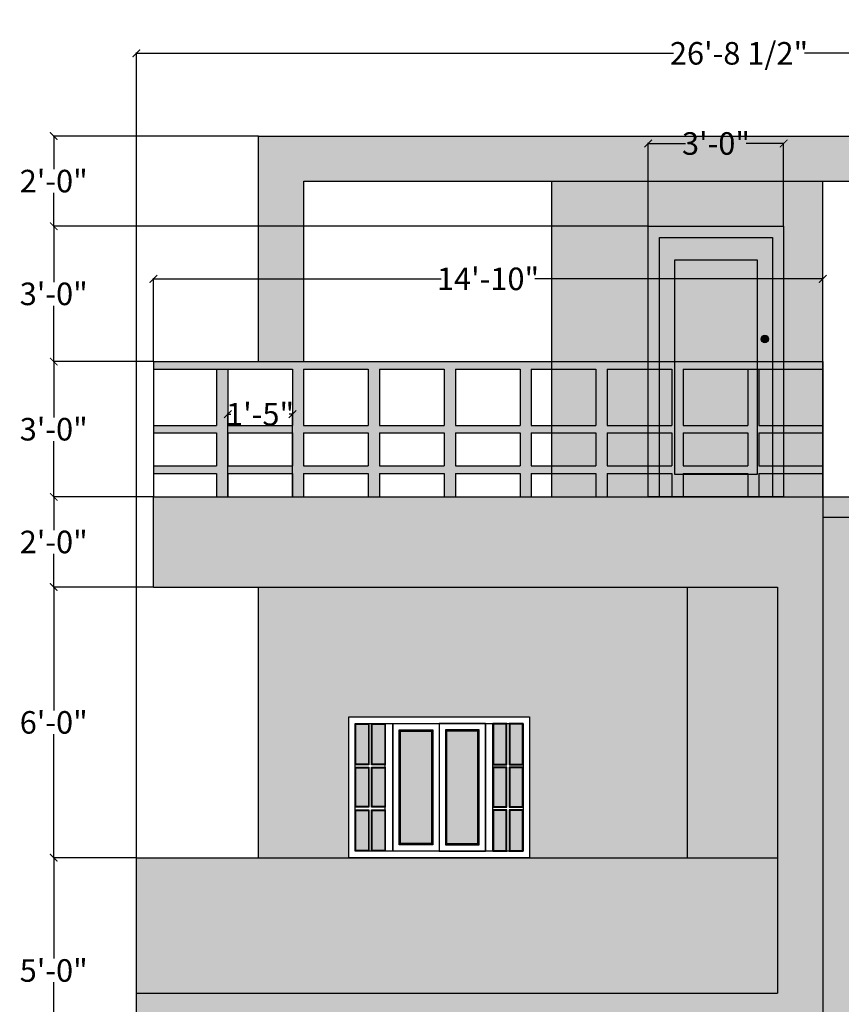
# Model space of a CAD drawing. Units: inches. Extents: x 528 to 2620, y -1066 to 798.
# Tile 40 of 41: x 2235 to 2453, y -891 to -629. Entities that reach past the tile are written whole.
import ezdxf

# ---------------------------------------------------------------- set-up
doc = ezdxf.new("R2010")
doc.units = ezdxf.units.IN
doc.header["$MEASUREMENT"] = 0
for name, color, linetype, lineweight in [('A-ANNO-DIMS', 2, 'Continuous', 18), ('A-ELEV', 7, 'Continuous', 25), ('A-ELEV-PATT', 8, 'Continuous', 13)]:
    doc.layers.add(name, color=color, linetype=linetype, lineweight=lineweight)
doc.styles.get("Standard").update_dxf_attribs({"font": 'arial.ttf'})
doc.dimstyles.get("Standard").update_dxf_attribs({"dimtxt": 6, "dimasz": 2, "dimexe": 0.18, "dimexo": 0.0625, "dimgap": 0.09, "dimtad": 0, "dimtih": 1, "dimtoh": 1, "dimdec": 1, "dimzin": 0, "dimdsep": 46, "dimlunit": 3, "dimtxsty": 'Standard', "dimblk": 'ARCHTICK', "dimcen": 0.09, "dimadec": 0, "dimazin": 0, "dimtfac": 1, "dimtdec": 1, "dimtofl": 0, "dimtmove": 0, "dimatfit": 3, "dimfxl": 1, "dimtolj": 1, "dimtzin": 0, "dimarcsym": 0})

# ---------------------------------------------------------------- blocks, each defined once
blk = doc.blocks.new('ww')
at = {"color": 0, "linetype": 'ByBlock'}
for p, q in [((30.67, -16.13), (126.65, -16.13)), ((30.67, -91.08), (30.67, -16.13)), ((34.01, -19.6), (123.32, -19.6)), ((34.01, -87.61), (34.01, -19.6)), ((34.01, -19.6), (49.87, -19.6)), ((34.01, -87.61), (34.01, -19.6)), ((50.03, -87.61), (50.03, -19.6)), ((54.03, -19.6), (54.03, -87.61)), ((103.29, -19.6), (103.29, -87.61)), ((107.29, -87.61), (107.29, -19.6)), ((123.32, -19.6), (123.32, -87.61)), ((126.65, -16.13), (126.65, -91.08)), ((123.32, -87.61), (34.01, -87.61)), ((126.65, -91.08), (30.67, -91.08))]:
    blk.add_line(p, q, dxfattribs=at)
at = {"color": 0, "linetype": 'ByBlock', "ltscale": 25}
for p, q in [((34.01, -41.58), (34.01, -19.6)), ((34.01, -19.6), (41.35, -19.6)), ((34.34, -41.23), (34.34, -19.95)), ((34.34, -19.95), (41.02, -19.95)), ((41.02, -19.95), (41.02, -41.23)), ((41.35, -19.6), (41.35, -41.58)), ((42.69, -41.58), (42.69, -19.6)), ((42.69, -19.6), (50.03, -19.6)), ((43.02, -41.23), (43.02, -19.95)), ((43.02, -19.95), (49.7, -19.95)), ((49.7, -19.95), (49.7, -41.23)), ((50.03, -19.6), (50.03, -41.58)), ((54.03, -87.61), (54.03, -19.6)), ((54.03, -19.6), (78.66, -19.6)), ((103.29, -19.6), (78.66, -19.6)), ((78.66, -19.6), (78.66, -87.61)), ((78.66, -19.6), (78.66, -87.61)), ((103.29, -87.61), (103.29, -19.6)), ((107.29, -19.6), (107.29, -41.58)), ((114.63, -19.6), (107.29, -19.6)), ((107.62, -19.95), (107.62, -41.23)), ((114.3, -19.95), (107.62, -19.95)), ((114.3, -41.23), (114.3, -19.95)), ((114.63, -41.58), (114.63, -19.6)), ((115.97, -19.6), (115.97, -41.58)), ((123.32, -19.6), (115.97, -19.6)), ((116.3, -19.95), (116.3, -41.23)), ((122.98, -19.95), (116.3, -19.95)), ((122.98, -41.23), (122.98, -19.95)), ((123.32, -41.58), (123.32, -19.6)), ((57.37, -84.14), (57.37, -23.07)), ((57.37, -23.07), (75.33, -23.07)), ((57.7, -83.8), (57.7, -23.42)), ((57.7, -23.42), (74.99, -23.42)), ((58.03, -83.45), (58.03, -23.77)), ((58.03, -23.77), (74.66, -23.77)), ((74.66, -23.77), (74.66, -83.45)), ((74.99, -23.42), (74.99, -83.8)), ((75.33, -23.07), (75.33, -84.14)), ((99.96, -23.07), (81.99, -23.07)), ((81.99, -23.07), (81.99, -84.14)), ((99.62, -23.42), (82.33, -23.42)), ((82.33, -23.42), (82.33, -83.8)), ((99.29, -23.77), (82.66, -23.77)), ((82.66, -23.77), (82.66, -83.45)), ((99.29, -83.45), (99.29, -23.77)), ((99.62, -83.8), (99.62, -23.42)), ((99.96, -84.14), (99.96, -23.07)), ((41.35, -41.58), (34.01, -41.58)), ((41.02, -41.23), (34.34, -41.23)), ((50.03, -41.58), (42.69, -41.58)), ((49.7, -41.23), (43.02, -41.23)), ((107.29, -41.58), (114.63, -41.58)), ((107.62, -41.23), (114.3, -41.23)), ((115.97, -41.58), (123.32, -41.58)), ((116.3, -41.23), (122.98, -41.23)), ((34.01, -64.25), (34.01, -42.97)), ((34.01, -42.97), (41.35, -42.97)), ((34.34, -63.9), (34.34, -43.31)), ((34.34, -43.31), (41.02, -43.31)), ((41.02, -43.31), (41.02, -63.9)), ((41.35, -42.97), (41.35, -64.25)), ((42.69, -64.25), (42.69, -42.97)), ((42.69, -42.97), (50.03, -42.97)), ((43.02, -63.9), (43.02, -43.31)), ((43.02, -43.31), (49.7, -43.31)), ((49.7, -43.31), (49.7, -63.9)), ((50.03, -42.97), (50.03, -64.25)), ((107.29, -42.97), (107.29, -64.25)), ((114.63, -42.97), (107.29, -42.97)), ((107.62, -43.31), (107.62, -63.9)), ((114.3, -43.31), (107.62, -43.31)), ((114.3, -63.9), (114.3, -43.31)), ((114.63, -64.25), (114.63, -42.97)), ((115.97, -42.97), (115.97, -64.25)), ((123.32, -42.97), (115.97, -42.97)), ((116.3, -43.31), (116.3, -63.9)), ((122.98, -43.31), (116.3, -43.31)), ((122.98, -63.9), (122.98, -43.31)), ((123.32, -64.25), (123.32, -42.97)), ((41.35, -64.25), (34.01, -64.25)), ((34.01, -87.61), (34.01, -65.64)), ((34.01, -65.64), (41.35, -65.64)), ((41.02, -63.9), (34.34, -63.9)), ((34.34, -87.27), (34.34, -65.98)), ((34.34, -65.98), (41.02, -65.98)), ((41.02, -65.98), (41.02, -87.27)), ((41.35, -65.64), (41.35, -87.61)), ((50.03, -64.25), (42.69, -64.25)), ((42.69, -87.61), (42.69, -65.64)), ((42.69, -65.64), (50.03, -65.64)), ((49.7, -63.9), (43.02, -63.9)), ((43.02, -87.27), (43.02, -65.98)), ((43.02, -65.98), (49.7, -65.98)), ((49.7, -65.98), (49.7, -87.27)), ((50.03, -65.64), (50.03, -87.61)), ((107.29, -64.25), (114.63, -64.25)), ((107.29, -65.64), (107.29, -87.61)), ((114.63, -65.64), (107.29, -65.64)), ((107.62, -63.9), (114.3, -63.9)), ((107.62, -65.98), (107.62, -87.27)), ((114.3, -65.98), (107.62, -65.98)), ((114.3, -87.27), (114.3, -65.98)), ((114.63, -87.61), (114.63, -65.64)), ((115.97, -64.25), (123.32, -64.25)), ((115.97, -65.64), (115.97, -87.61)), ((123.32, -65.64), (115.97, -65.64)), ((116.3, -63.9), (122.98, -63.9)), ((116.3, -65.98), (116.3, -87.27)), ((122.98, -65.98), (116.3, -65.98)), ((122.98, -87.27), (122.98, -65.98)), ((123.32, -87.61), (123.32, -65.64)), ((74.99, -83.8), (57.7, -83.8)), ((74.66, -83.45), (58.03, -83.45)), ((82.33, -83.8), (99.62, -83.8)), ((82.66, -83.45), (99.29, -83.45)), ((41.35, -87.61), (34.01, -87.61)), ((41.02, -87.27), (34.34, -87.27)), ((50.03, -87.61), (42.69, -87.61)), ((49.7, -87.27), (43.02, -87.27)), ((78.66, -87.61), (54.03, -87.61)), ((75.33, -84.14), (57.37, -84.14)), ((78.66, -87.61), (103.29, -87.61)), ((81.99, -84.14), (99.96, -84.14)), ((107.29, -87.61), (114.63, -87.61)), ((107.62, -87.27), (114.3, -87.27)), ((115.97, -87.61), (123.32, -87.61)), ((116.3, -87.27), (122.98, -87.27))]:
    blk.add_line(p, q, dxfattribs=at)
blk = doc.blocks.new('*U24')
blk.add_lwpolyline([(3.12, 0.01), (0.12, 0.01), (0.12, 72.01), (36.12, 72.01), (36.12, 0.01), (33.12, 0.01)])
for points in [[(33.12, 68.99), (33.12, 0.01), (3.12, 0.01), (3.12, 68.99)], [(29.12, 6.01), (29.12, 62.99), (7.12, 62.99), (7.12, 6.01)]]:
    blk.add_lwpolyline(points, close=True)
blk.add_circle((31.12, 42.01), 1)
blk = doc.blocks.new('_ArchTick')
at = {"color": 0, "linetype": 'ByBlock', "const_width": 0.15}
blk.add_lwpolyline([(-0.5, -0.5), (0.5, 0.5)], dxfattribs=at)
blk = doc.blocks.new('*D70')
at = {"layer": 'A-ANNO-DIMS', "color": 0, "lineweight": -2, "transparency": 16777216}
for p, q in [((2266.05, -852.09), (2266.05, -637.97)), ((2266.05, -638.15), (2408.86, -638.15)), ((2586.55, -638.15), (2443.73, -638.15)), ((2586.55, -660.09), (2586.55, -637.97))]:
    blk.add_line(p, q, dxfattribs=at)
at = {"layer": 'Defpoints', "color": 0, "transparency": 16777216}
for p in [(2586.55, -638.15), (2586.55, -660.15), (2266.05, -852.15)]:
    blk.add_point(p, dxfattribs=at)
at = {"layer": 'A-ANNO-DIMS', "color": 0, "lineweight": -2, "transparency": 16777216, "xscale": 2, "yscale": 2, "zscale": 2, "rotation": 180}
blk.add_blockref('_ArchTick', (2266.05, -638.15), dxfattribs=at)
at = {"layer": 'A-ANNO-DIMS', "color": 0, "lineweight": -2, "transparency": 16777216, "xscale": 2, "yscale": 2, "zscale": 2}
blk.add_blockref('_ArchTick', (2586.55, -638.15), dxfattribs=at)
at = {"layer": 'A-ANNO-DIMS', "color": 0, "transparency": 16777216, "insert": (2426.3, -638.15), "char_height": 6, "attachment_point": 5}
blk.add_mtext('\\A1;26\'-8 1/2"', dxfattribs=at)
blk = doc.blocks.new('*D74')
at = {"layer": 'A-ANNO-DIMS', "color": 0, "lineweight": -2, "transparency": 16777216}
for p, q in [((2265.98, -852.15), (2243.87, -852.15)), ((2244.05, -852.15), (2244.05, -878.99)), ((2244.05, -912.15), (2244.05, -885.3)), ((2265.98, -912.15), (2243.87, -912.15))]:
    blk.add_line(p, q, dxfattribs=at)
at = {"layer": 'Defpoints', "color": 0, "transparency": 16777216}
for p in [(2244.05, -852.15), (2266.05, -852.15), (2266.05, -912.15)]:
    blk.add_point(p, dxfattribs=at)
at = {"layer": 'A-ANNO-DIMS', "color": 0, "lineweight": -2, "transparency": 16777216, "xscale": 2, "yscale": 2, "zscale": 2}
for p, rotation in [((2244.05, -852.15), 90), ((2244.05, -912.15), 270)]:
    blk.add_blockref('_ArchTick', p, dxfattribs=dict(at, rotation=rotation))
at = {"layer": 'A-ANNO-DIMS', "color": 0, "transparency": 16777216, "insert": (2244.05, -882.15), "char_height": 6, "attachment_point": 5}
blk.add_mtext('\\A1;5\'-0"', dxfattribs=at)
blk = doc.blocks.new('*D75')
at = {"layer": 'A-ANNO-DIMS', "color": 0, "lineweight": -2, "transparency": 16777216}
for p, q in [((2270.48, -780.15), (2243.87, -780.15)), ((2244.05, -780.15), (2244.05, -812.99)), ((2244.05, -852.15), (2244.05, -819.3)), ((2265.98, -852.15), (2243.87, -852.15))]:
    blk.add_line(p, q, dxfattribs=at)
at = {"layer": 'Defpoints', "color": 0, "transparency": 16777216}
for p in [(2244.05, -780.15), (2270.55, -780.15), (2266.05, -852.15)]:
    blk.add_point(p, dxfattribs=at)
at = {"layer": 'A-ANNO-DIMS', "color": 0, "lineweight": -2, "transparency": 16777216, "xscale": 2, "yscale": 2, "zscale": 2}
for p, rotation in [((2244.05, -780.15), 90), ((2244.05, -852.15), 270)]:
    blk.add_blockref('_ArchTick', p, dxfattribs=dict(at, rotation=rotation))
at = {"layer": 'A-ANNO-DIMS', "color": 0, "transparency": 16777216, "insert": (2244.05, -816.15), "char_height": 6, "attachment_point": 5}
blk.add_mtext('\\A1;6\'-0"', dxfattribs=at)
blk = doc.blocks.new('*D76')
at = {"layer": 'A-ANNO-DIMS', "color": 0, "lineweight": -2, "transparency": 16777216}
for p, q in [((2270.48, -756.15), (2243.87, -756.15)), ((2244.05, -756.15), (2244.05, -764.99)), ((2244.05, -780.15), (2244.05, -771.3)), ((2270.48, -780.15), (2243.87, -780.15))]:
    blk.add_line(p, q, dxfattribs=at)
at = {"layer": 'Defpoints', "color": 0, "transparency": 16777216}
for p in [(2244.05, -756.15), (2270.55, -756.15), (2270.55, -780.15)]:
    blk.add_point(p, dxfattribs=at)
at = {"layer": 'A-ANNO-DIMS', "color": 0, "lineweight": -2, "transparency": 16777216, "xscale": 2, "yscale": 2, "zscale": 2}
for p, rotation in [((2244.05, -756.15), 90), ((2244.05, -780.15), 270)]:
    blk.add_blockref('_ArchTick', p, dxfattribs=dict(at, rotation=rotation))
at = {"layer": 'A-ANNO-DIMS', "color": 0, "transparency": 16777216, "insert": (2244.05, -768.15), "char_height": 6, "attachment_point": 5}
blk.add_mtext('\\A1;2\'-0"', dxfattribs=at)
blk = doc.blocks.new('*D77')
at = {"layer": 'A-ANNO-DIMS', "color": 0, "lineweight": -2, "transparency": 16777216}
for p, q in [((2270.48, -720.15), (2243.87, -720.15)), ((2244.05, -720.15), (2244.05, -734.99)), ((2244.05, -756.15), (2244.05, -741.3)), ((2270.48, -756.15), (2243.87, -756.15))]:
    blk.add_line(p, q, dxfattribs=at)
at = {"layer": 'Defpoints', "color": 0, "transparency": 16777216}
for p in [(2244.05, -720.15), (2270.55, -720.15), (2270.55, -756.15)]:
    blk.add_point(p, dxfattribs=at)
at = {"layer": 'A-ANNO-DIMS', "color": 0, "lineweight": -2, "transparency": 16777216, "xscale": 2, "yscale": 2, "zscale": 2}
for p, rotation in [((2244.05, -720.15), 90), ((2244.05, -756.15), 270)]:
    blk.add_blockref('_ArchTick', p, dxfattribs=dict(at, rotation=rotation))
at = {"layer": 'A-ANNO-DIMS', "color": 0, "transparency": 16777216, "insert": (2244.05, -738.15), "char_height": 6, "attachment_point": 5}
blk.add_mtext('\\A1;3\'-0"', dxfattribs=at)
blk = doc.blocks.new('*D78')
at = {"layer": 'A-ANNO-DIMS', "color": 0, "lineweight": -2, "transparency": 16777216}
for p, q in [((2402.11, -684.14), (2243.87, -684.14)), ((2244.05, -684.14), (2244.05, -698.99)), ((2244.05, -720.15), (2244.05, -705.3)), ((2270.48, -720.15), (2243.87, -720.15))]:
    blk.add_line(p, q, dxfattribs=at)
at = {"layer": 'Defpoints', "color": 0, "transparency": 16777216}
for p in [(2244.05, -684.14), (2402.17, -684.14), (2270.55, -720.15)]:
    blk.add_point(p, dxfattribs=at)
at = {"layer": 'A-ANNO-DIMS', "color": 0, "lineweight": -2, "transparency": 16777216, "xscale": 2, "yscale": 2, "zscale": 2}
for p, rotation in [((2244.05, -684.14), 90), ((2244.05, -720.15), 270)]:
    blk.add_blockref('_ArchTick', p, dxfattribs=dict(at, rotation=rotation))
at = {"layer": 'A-ANNO-DIMS', "color": 0, "transparency": 16777216, "insert": (2244.05, -702.14), "char_height": 6, "attachment_point": 5}
blk.add_mtext('\\A1;3\'-0"', dxfattribs=at)
blk = doc.blocks.new('*D79')
at = {"layer": 'A-ANNO-DIMS', "color": 0, "lineweight": -2, "transparency": 16777216}
for p, q in [((2298.48, -660.15), (2243.87, -660.15)), ((2244.05, -660.15), (2244.05, -668.99)), ((2244.05, -684.14), (2244.05, -675.3)), ((2402.11, -684.14), (2243.87, -684.14))]:
    blk.add_line(p, q, dxfattribs=at)
at = {"layer": 'Defpoints', "color": 0, "transparency": 16777216}
for p in [(2244.05, -660.15), (2298.55, -660.15), (2402.17, -684.14)]:
    blk.add_point(p, dxfattribs=at)
at = {"layer": 'A-ANNO-DIMS', "color": 0, "lineweight": -2, "transparency": 16777216, "xscale": 2, "yscale": 2, "zscale": 2}
for p, rotation in [((2244.05, -660.15), 90), ((2244.05, -684.14), 270)]:
    blk.add_blockref('_ArchTick', p, dxfattribs=dict(at, rotation=rotation))
at = {"layer": 'A-ANNO-DIMS', "color": 0, "transparency": 16777216, "insert": (2244.05, -672.14), "char_height": 6, "attachment_point": 5}
blk.add_mtext('\\A1;2\'-0"', dxfattribs=at)
blk = doc.blocks.new('*D88')
at = {"layer": 'A-ANNO-DIMS', "color": 0, "lineweight": -2, "transparency": 16777216}
for p, q in [((2270.55, -720.09), (2270.55, -697.97)), ((2270.55, -698.15), (2347.1, -698.15)), ((2448.55, -698.15), (2371.99, -698.15)), ((2448.55, -720.09), (2448.55, -697.97))]:
    blk.add_line(p, q, dxfattribs=at)
at = {"layer": 'Defpoints', "color": 0, "transparency": 16777216}
for p in [(2448.55, -698.15), (2270.55, -720.15), (2448.55, -720.15)]:
    blk.add_point(p, dxfattribs=at)
at = {"layer": 'A-ANNO-DIMS', "color": 0, "lineweight": -2, "transparency": 16777216, "xscale": 2, "yscale": 2, "zscale": 2, "rotation": 180}
blk.add_blockref('_ArchTick', (2270.55, -698.15), dxfattribs=at)
at = {"layer": 'A-ANNO-DIMS', "color": 0, "lineweight": -2, "transparency": 16777216, "xscale": 2, "yscale": 2, "zscale": 2}
blk.add_blockref('_ArchTick', (2448.55, -698.15), dxfattribs=at)
at = {"layer": 'A-ANNO-DIMS', "color": 0, "transparency": 16777216, "insert": (2359.55, -698.15), "char_height": 6, "attachment_point": 5}
blk.add_mtext('\\A1;14\'-10"', dxfattribs=at)
blk = doc.blocks.new('*D90')
at = {"layer": 'A-ANNO-DIMS', "color": 0, "lineweight": -2, "transparency": 16777216}
for p, q in [((2402.17, -684.07), (2402.17, -661.96)), ((2402.17, -662.14), (2412.11, -662.14)), ((2438.17, -662.14), (2428.24, -662.14)), ((2438.17, -684.07), (2438.17, -661.96))]:
    blk.add_line(p, q, dxfattribs=at)
at = {"layer": 'Defpoints', "color": 0, "transparency": 16777216}
for p in [(2438.17, -662.14), (2402.17, -684.14), (2438.17, -684.14)]:
    blk.add_point(p, dxfattribs=at)
at = {"layer": 'A-ANNO-DIMS', "color": 0, "lineweight": -2, "transparency": 16777216, "xscale": 2, "yscale": 2, "zscale": 2, "rotation": 180}
blk.add_blockref('_ArchTick', (2402.17, -662.14), dxfattribs=at)
at = {"layer": 'A-ANNO-DIMS', "color": 0, "lineweight": -2, "transparency": 16777216, "xscale": 2, "yscale": 2, "zscale": 2}
blk.add_blockref('_ArchTick', (2438.17, -662.14), dxfattribs=at)
at = {"layer": 'A-ANNO-DIMS', "color": 0, "transparency": 16777216, "insert": (2420.17, -662.14), "char_height": 6, "attachment_point": 5}
blk.add_mtext('\\A1;3\'-0"', dxfattribs=at)
blk = doc.blocks.new('*D91')
at = {"layer": 'A-ANNO-DIMS', "color": 0, "lineweight": -2, "transparency": 16777216}
for p, q in [((2290.34, -756.09), (2290.34, -733.97)), ((2290.34, -734.15), (2291.15, -734.15)), ((2307.52, -734.15), (2306.71, -734.15)), ((2307.52, -756.09), (2307.52, -733.97))]:
    blk.add_line(p, q, dxfattribs=at)
at = {"layer": 'Defpoints', "color": 0, "transparency": 16777216}
for p in [(2307.52, -734.15), (2290.34, -756.15), (2307.52, -756.15)]:
    blk.add_point(p, dxfattribs=at)
at = {"layer": 'A-ANNO-DIMS', "color": 0, "lineweight": -2, "transparency": 16777216, "xscale": 2, "yscale": 2, "zscale": 2, "rotation": 180}
blk.add_blockref('_ArchTick', (2290.34, -734.15), dxfattribs=at)
at = {"layer": 'A-ANNO-DIMS', "color": 0, "lineweight": -2, "transparency": 16777216, "xscale": 2, "yscale": 2, "zscale": 2}
blk.add_blockref('_ArchTick', (2307.52, -734.15), dxfattribs=at)
at = {"layer": 'A-ANNO-DIMS', "color": 0, "transparency": 16777216, "insert": (2298.93, -734.15), "char_height": 6, "attachment_point": 5}
blk.add_mtext('\\A1;1\'-5"', dxfattribs=at)

msp = doc.modelspace()

# ---------------------------------------------------------------- hatches: boundary and pattern name
at = {"layer": 'A-ELEV-PATT', "transparency": 33554687}
h = msp.add_hatch(color=256, dxfattribs=at)
h.dxf.hatch_style = 1
h.paths.add_polyline_path([(2586.55, -660.15), (2298.55, -660.15), (2298.55, -720.15), (2310.55, -720.15), (2310.55, -672.15), (2562.55, -672.15), (2562.55, -900.15), (2448.55, -900.15), (2448.55, -912.15), (2586.55, -912.15)])
h = msp.add_hatch(color=256, dxfattribs=at)
h.dxf.hatch_style = 1
h.paths.add_polyline_path([(2402.17, -684.14), (2438.17, -684.14), (2438.17, -720.15), (2448.55, -720.15), (2448.55, -672.15), (2376.55, -672.15), (2376.55, -720.15), (2402.17, -720.15)])
h.paths.add_polyline_path([(2402.17, -722.15), (2391.24, -722.15), (2391.24, -737.15), (2402.17, -737.15)])
h.paths.add_polyline_path([(2388.24, -722.15), (2376.55, -722.15), (2376.55, -737.15), (2388.24, -737.15)])
h.paths.add_polyline_path([(2388.24, -739.15), (2376.55, -739.15), (2376.55, -747.92), (2388.24, -747.92)])
h.paths.add_polyline_path([(2402.17, -739.15), (2391.24, -739.15), (2391.24, -747.92), (2402.17, -747.92)])
h.paths.add_polyline_path([(2388.24, -749.92), (2376.55, -749.92), (2376.55, -756.15), (2388.24, -756.15)])
h.paths.add_polyline_path([(2402.17, -749.92), (2391.24, -749.92), (2391.24, -756.15), (2402.17, -756.15)])
h.paths.add_polyline_path([(2448.55, -749.92), (2438.17, -749.92), (2438.17, -756.15), (2448.55, -756.15)])
h.paths.add_polyline_path([(2448.55, -739.15), (2438.17, -739.15), (2438.17, -747.92), (2448.55, -747.92)])
h.paths.add_polyline_path([(2448.55, -722.15), (2438.17, -722.15), (2438.17, -737.15), (2448.55, -737.15)])
h = msp.add_hatch(color=256, dxfattribs=at)
h.dxf.hatch_style = 1
h.paths.add_polyline_path([(2431.17, -693.16), (2409.17, -693.16), (2409.17, -720.15), (2431.17, -720.15)], flags=16)
h.paths.add_polyline_path([(2428.6, -739.15), (2411.42, -739.15), (2411.42, -747.92), (2428.6, -747.92)], flags=0)
h.paths.add_polyline_path([(2428.6, -722.15), (2411.42, -722.15), (2411.42, -737.15), (2428.6, -737.15)], flags=0)
h.paths.add_polyline_path([(2408.42, -722.15), (2405.17, -722.15), (2405.17, -737.15), (2408.42, -737.15)], flags=17)
h.paths.add_polyline_path([(2408.42, -739.15), (2405.17, -739.15), (2405.17, -747.92), (2408.42, -747.92)], flags=16)
h.paths.add_polyline_path([(2408.42, -749.92), (2405.17, -749.92), (2405.17, -756.14), (2408.42, -756.14)], flags=16)
h.paths.add_polyline_path([(2405.17, -749.92), (2402.17, -749.92), (2402.17, -756.14), (2405.17, -756.14)])
h.paths.add_polyline_path([(2405.17, -739.15), (2402.17, -739.15), (2402.17, -747.92), (2405.17, -747.92)])
h.paths.add_polyline_path([(2405.17, -722.15), (2402.17, -722.15), (2402.17, -737.15), (2405.17, -737.15)])
h.paths.add_polyline_path([(2435.17, -687.16), (2405.17, -687.16), (2405.17, -722.15), (2408.42, -722.15), (2408.42, -737.15), (2405.17, -737.15), (2405.17, -756.14), (2435.17, -756.14)])
h.paths.add_polyline_path([(2409.17, -693.16), (2431.17, -693.16), (2431.17, -750.14), (2409.17, -750.14)], flags=16)
h.paths.add_polyline_path([(2434.17, -714.14, -1), (2432.17, -714.14, -1)], flags=16)
h.paths.add_polyline_path([(2411.42, -739.15), (2428.6, -739.15), (2428.6, -747.92), (2411.42, -747.92)], flags=0)
h.paths.add_polyline_path([(2405.17, -687.16), (2435.17, -687.16), (2435.17, -720.15), (2438.17, -720.15), (2438.17, -684.14), (2402.17, -684.14), (2402.17, -720.15), (2405.17, -720.15)])
h = msp.add_hatch(color=256, dxfattribs=at)
h.dxf.hatch_style = 1
h.paths.add_polyline_path([(2431.17, -693.16), (2409.17, -693.16), (2409.17, -750.14), (2431.17, -750.14)], flags=0)
h.paths.add_polyline_path([(2435.17, -687.16), (2405.17, -687.16), (2405.17, -756.14), (2435.17, -756.14)], flags=17)
h.paths.add_polyline_path([(2431.17, -750.14), (2409.17, -750.14), (2409.17, -693.16), (2431.17, -693.16)], flags=16)
h.paths.add_polyline_path([(2432.17, -714.14, -1), (2434.17, -714.14, -1)], flags=16)
h.paths.add_polyline_path([(2438.17, -684.14), (2402.17, -684.14), (2402.17, -756.14), (2405.17, -756.14), (2405.17, -687.16), (2435.17, -687.16), (2435.17, -756.14), (2438.17, -756.14)])
h = msp.add_hatch(color=256, dxfattribs=at)
h.dxf.hatch_style = 1
h.paths.add_polyline_path([(2431.17, -693.16), (2409.17, -693.16), (2409.17, -750.14), (2431.17, -750.14)])
h = msp.add_hatch(color=256, dxfattribs=at)
h.dxf.hatch_style = 1
h.paths.add_polyline_path([(2434.17, -714.14, 1), (2432.17, -714.14, 1)])
at = {"layer": 'A-ELEV-PATT', "transparency": 33554536}
h = msp.add_hatch(color=256, dxfattribs=at)
h.dxf.hatch_style = 1
h.paths.add_polyline_path([(2411.42, -722.15), (2448.55, -722.15), (2448.55, -720.15), (2270.55, -720.15), (2270.55, -722.15), (2307.52, -722.15), (2307.52, -737.15), (2290.34, -737.15), (2290.34, -722.15), (2287.34, -722.15), (2287.34, -737.15), (2270.55, -737.15), (2270.55, -739.15), (2287.34, -739.15), (2287.34, -747.92), (2270.55, -747.92), (2270.55, -749.92), (2287.34, -749.92), (2287.34, -756.15), (2290.34, -756.15), (2290.34, -749.92), (2307.52, -749.92), (2307.52, -756.15), (2310.52, -756.15), (2310.52, -749.92), (2327.7, -749.92), (2327.7, -756.15), (2330.7, -756.15), (2330.7, -749.92), (2347.88, -749.92), (2347.88, -756.15), (2350.88, -756.15), (2350.88, -749.92), (2368.06, -749.92), (2368.06, -756.15), (2371.06, -756.15), (2371.06, -749.92), (2388.24, -749.92), (2388.24, -756.15), (2391.24, -756.15), (2391.24, -749.92), (2408.42, -749.92), (2408.42, -756.15), (2411.42, -756.15), (2411.42, -749.92), (2428.6, -749.92), (2428.6, -756.15), (2431.6, -756.15), (2431.6, -749.92), (2448.55, -749.92), (2448.55, -747.92), (2431.6, -747.92), (2431.6, -739.15), (2448.55, -739.15), (2448.55, -737.15), (2431.6, -737.15), (2431.6, -722.15), (2428.6, -722.15), (2428.6, -737.15), (2411.42, -737.15)])
h.paths.add_polyline_path([(2327.7, -737.15), (2310.52, -737.15), (2310.52, -722.15), (2327.7, -722.15)], flags=16)
h.paths.add_polyline_path([(2330.7, -737.15), (2330.7, -722.15), (2347.88, -722.15), (2347.88, -737.15)], flags=16)
h.paths.add_polyline_path([(2327.7, -739.15), (2327.7, -747.92), (2310.52, -747.92), (2310.52, -739.15)], flags=16)
h.paths.add_polyline_path([(2330.7, -739.15), (2347.88, -739.15), (2347.88, -747.92), (2330.7, -747.92)], flags=16)
h.paths.add_polyline_path([(2307.52, -739.15), (2307.52, -747.92), (2290.34, -747.92), (2290.34, -739.15)], flags=16)
h.paths.add_polyline_path([(2350.88, -737.15), (2350.88, -722.15), (2368.06, -722.15), (2368.06, -737.15)], flags=16)
h.paths.add_polyline_path([(2350.88, -739.15), (2368.06, -739.15), (2368.06, -747.92), (2350.88, -747.92)], flags=16)
h.paths.add_polyline_path([(2371.06, -737.15), (2371.06, -722.15), (2388.24, -722.15), (2388.24, -737.15)], flags=16)
h.paths.add_polyline_path([(2371.06, -739.15), (2388.24, -739.15), (2388.24, -747.92), (2371.06, -747.92)], flags=16)
h.paths.add_polyline_path([(2391.24, -737.15), (2391.24, -722.15), (2408.42, -722.15), (2408.42, -737.15)], flags=16)
h.paths.add_polyline_path([(2391.24, -739.15), (2408.42, -739.15), (2408.42, -747.92), (2391.24, -747.92)], flags=16)
h.paths.add_polyline_path([(2411.42, -739.15), (2428.6, -739.15), (2428.6, -747.92), (2411.42, -747.92)], flags=16)
at = {"layer": 'A-ELEV-PATT', "transparency": 33554687}
h = msp.add_hatch(color=256, dxfattribs=at)
h.dxf.hatch_style = 1
h.paths.add_polyline_path([(2448.55, -756.15), (2270.55, -756.15), (2270.55, -780.15), (2436.55, -780.15), (2436.55, -888.15), (2266.05, -888.15), (2266.05, -912.15), (2448.55, -912.15)])
h = msp.add_hatch(color=256, dxfattribs=at)
h.dxf.hatch_style = 1
h.paths.add_polyline_path([(2562.55, -756.15), (2448.55, -756.15), (2448.55, -761.55), (2562.55, -761.55)])
h = msp.add_hatch(color=256, dxfattribs=at)
h.dxf.hatch_style = 1
h.paths.add_polyline_path([(2586.55, -912.15), (2448.55, -912.15), (2448.55, -940.66), (2547.55, -940.66), (2547.55, -990.15), (2448.55, -990.15), (2448.55, -1020.15), (2586.55, -1020.15)])
h.paths.add_polyline_path([(2481.55, -789.84), (2562.55, -789.84), (2562.55, -761.55), (2448.55, -761.55), (2448.55, -900.15), (2562.55, -900.15), (2562.55, -876.97), (2481.55, -876.97), (2481.55, -833.41)])
h.paths.add_polyline_path([(2412.55, -780.15), (2298.55, -780.15), (2298.55, -852.15), (2322.55, -852.15), (2322.55, -814.66), (2370.55, -814.66), (2370.55, -852.15), (2412.55, -852.15)])
h.paths.add_polyline_path([(2394.55, -940.36), (2442.55, -940.36), (2442.55, -1020.15), (2448.55, -1020.15), (2448.55, -990.15), (2448.55, -912.15), (2310.55, -912.15), (2310.55, -1020.15), (2394.55, -1020.15)])
h.paths.add_polyline_path([(2327.05, -984.15), (2327.05, -946.66), (2375.05, -946.66), (2375.05, -984.15)], flags=16)
h.paths.add_polyline_path([(2328.71, -982.41), (2328.71, -948.4), (2336.65, -948.4), (2336.73, -948.4), (2373.38, -948.4), (2373.38, -982.41), (2369.7, -982.41)], flags=0)
h.paths.add_polyline_path([(2338.73, -982.41), (2338.73, -948.4), (2351.05, -948.4), (2363.36, -948.4), (2363.36, -982.41), (2351.05, -982.41)], flags=0)
h.paths.add_polyline_path([(2340.4, -980.68), (2340.4, -950.13), (2349.38, -950.13), (2349.38, -980.68)], flags=0)
h.paths.add_polyline_path([(2340.73, -980.33), (2340.73, -950.48), (2349.05, -950.48), (2349.05, -980.33)], flags=0)
h.paths.add_polyline_path([(2352.71, -980.68), (2352.71, -950.13), (2361.7, -950.13), (2361.7, -980.68)], flags=0)
h.paths.add_polyline_path([(2353.05, -980.33), (2353.05, -950.48), (2361.36, -950.48), (2361.36, -980.33)], flags=0)
h.paths.add_polyline_path([(2336.73, -982.41), (2333.05, -982.41), (2333.05, -971.42), (2336.73, -971.42), (2336.73, -970.73), (2333.05, -970.73), (2333.05, -960.08), (2336.73, -960.08), (2336.73, -959.39), (2333.05, -959.39), (2333.05, -948.57), (2336.73, -948.57)], flags=0)
h.paths.add_polyline_path([(2333.22, -982.24), (2333.22, -971.6), (2336.73, -971.6), (2336.73, -982.24)], flags=0)
h.paths.add_polyline_path([(2332.39, -982.41), (2328.71, -982.41), (2328.71, -948.4), (2332.39, -948.4), (2332.39, -959.39), (2328.71, -959.39), (2328.71, -960.08), (2332.39, -960.08), (2332.39, -970.73), (2328.71, -970.73), (2328.71, -971.42), (2332.39, -971.42)], flags=0)
h.paths.add_polyline_path([(2332.22, -982.24), (2328.71, -982.24), (2328.71, -971.6), (2332.22, -971.6)], flags=0)
h.paths.add_polyline_path([(2365.36, -982.41), (2365.36, -948.4), (2369.04, -948.4), (2369.04, -959.39), (2365.36, -959.39), (2365.36, -960.08), (2369.04, -960.08), (2369.04, -970.73), (2365.36, -970.73), (2365.36, -971.42), (2369.04, -971.42), (2369.04, -982.41)], flags=0)
h.paths.add_polyline_path([(2369.7, -971.42), (2373.38, -971.42), (2373.38, -982.24), (2369.7, -982.24)], flags=0)
h.paths.add_polyline_path([(2333.22, -970.55), (2333.22, -960.26), (2336.73, -960.26), (2336.73, -970.55)], flags=0)
h.paths.add_polyline_path([(2332.22, -970.55), (2328.71, -970.55), (2328.71, -960.26), (2332.22, -960.26)], flags=0)
h.paths.add_polyline_path([(2369.7, -970.73), (2369.7, -960.08), (2373.38, -960.08), (2373.38, -970.73)], flags=0)
h.paths.add_polyline_path([(2336.56, -959.22), (2336.56, -948.57), (2336.73, -948.4), (2336.73, -959.22)], flags=0)
h.paths.add_polyline_path([(2332.22, -959.22), (2328.71, -959.22), (2328.71, -948.57), (2332.22, -948.57)], flags=0)
h.paths.add_polyline_path([(2369.7, -959.39), (2369.7, -948.4), (2373.38, -948.4), (2373.38, -959.39)], flags=0)
h = msp.add_hatch(color=256, dxfattribs=at)
h.dxf.hatch_style = 1
h.paths.add_polyline_path([(2436.55, -780.15), (2412.55, -780.15), (2412.55, -852.15), (2436.55, -852.15)])
h = msp.add_hatch(color=256, dxfattribs=at)
h.dxf.hatch_style = 1
h.paths.add_polyline_path([(2527.86, -818.48), (2519.55, -818.48), (2519.55, -848.33), (2527.86, -848.33)])
h.paths.add_polyline_path([(2515.55, -818.48), (2507.23, -818.48), (2507.23, -848.33), (2515.55, -848.33)])
h.paths.add_polyline_path([(2498.72, -816.57), (2495.38, -816.57), (2495.38, -827.22), (2498.72, -827.22)])
h.paths.add_polyline_path([(2503.06, -816.57), (2499.72, -816.57), (2499.72, -827.22), (2503.06, -827.22)])
h.paths.add_polyline_path([(2498.72, -828.26), (2495.38, -828.26), (2495.38, -838.55), (2498.72, -838.55)])
h.paths.add_polyline_path([(2503.06, -828.26), (2499.72, -828.26), (2499.72, -838.55), (2503.06, -838.55)])
h.paths.add_polyline_path([(2498.72, -839.6), (2495.38, -839.6), (2495.38, -850.24), (2498.72, -850.24)])
h.paths.add_polyline_path([(2503.06, -839.6), (2499.72, -839.6), (2499.72, -850.24), (2503.06, -850.24)])
h.paths.add_polyline_path([(2535.37, -839.6), (2532.03, -839.6), (2532.03, -850.24), (2535.37, -850.24)])
h.paths.add_polyline_path([(2539.71, -839.6), (2536.37, -839.6), (2536.37, -850.24), (2539.71, -850.24)])
h.paths.add_polyline_path([(2535.37, -828.26), (2532.03, -828.26), (2532.03, -838.55), (2535.37, -838.55)])
h.paths.add_polyline_path([(2539.71, -828.26), (2536.37, -828.26), (2536.37, -838.55), (2539.71, -838.55)])
h.paths.add_polyline_path([(2535.37, -816.57), (2532.03, -816.57), (2532.03, -827.22), (2535.37, -827.22)])
h.paths.add_polyline_path([(2356.86, -818.48), (2348.55, -818.48), (2348.55, -848.33), (2356.86, -848.33)])
h.paths.add_polyline_path([(2344.55, -818.48), (2336.23, -818.48), (2336.23, -848.33), (2344.55, -848.33)])
h.paths.add_polyline_path([(2327.72, -816.57), (2324.38, -816.57), (2324.38, -827.22), (2327.72, -827.22)])
h.paths.add_polyline_path([(2332.06, -816.57), (2328.72, -816.57), (2328.72, -827.22), (2332.06, -827.22)])
h.paths.add_polyline_path([(2327.72, -828.26), (2324.38, -828.26), (2324.38, -838.55), (2327.72, -838.55)])
h.paths.add_polyline_path([(2332.06, -828.26), (2328.72, -828.26), (2328.72, -838.55), (2332.06, -838.55)])
h.paths.add_polyline_path([(2327.72, -839.6), (2324.38, -839.6), (2324.38, -850.24), (2327.72, -850.24)])
h.paths.add_polyline_path([(2332.06, -839.6), (2328.72, -839.6), (2328.72, -850.24), (2332.06, -850.24)])
h.paths.add_polyline_path([(2368.71, -839.6), (2365.37, -839.6), (2365.37, -850.24), (2368.71, -850.24)])
h.paths.add_polyline_path([(2364.37, -839.6), (2361.03, -839.6), (2361.03, -850.24), (2364.37, -850.24)])
h.paths.add_polyline_path([(2364.37, -828.26), (2361.03, -828.26), (2361.03, -838.55), (2364.37, -838.55)])
h.paths.add_polyline_path([(2368.71, -828.26), (2365.37, -828.26), (2365.37, -838.55), (2368.71, -838.55)])
h.paths.add_polyline_path([(2364.37, -816.57), (2361.03, -816.57), (2361.03, -827.22), (2364.37, -827.22)])
h.paths.add_polyline_path([(2368.71, -816.57), (2365.37, -816.57), (2365.37, -827.22), (2368.71, -827.22)])
h.paths.add_polyline_path([(2361.36, -950.48), (2353.05, -950.48), (2353.05, -980.33), (2361.36, -980.33)])
h.paths.add_polyline_path([(2349.05, -950.48), (2340.73, -950.48), (2340.73, -980.33), (2349.05, -980.33)])
h.paths.add_polyline_path([(2336.56, -971.6), (2333.22, -971.6), (2333.22, -982.24), (2336.56, -982.24)])
h.paths.add_polyline_path([(2332.22, -971.6), (2328.88, -971.6), (2328.88, -982.24), (2332.22, -982.24)])
h.paths.add_polyline_path([(2336.56, -960.26), (2333.22, -960.26), (2333.22, -970.55), (2336.56, -970.55)])
h.paths.add_polyline_path([(2332.22, -960.26), (2328.88, -960.26), (2328.88, -970.55), (2332.22, -970.55)])
h.paths.add_polyline_path([(2332.22, -948.57), (2328.88, -948.57), (2328.88, -959.22), (2332.22, -959.22)])
h.paths.add_polyline_path([(2336.56, -948.57), (2333.22, -948.57), (2333.22, -959.22), (2336.56, -959.22)])
h.paths.add_polyline_path([(2368.87, -971.6), (2365.53, -971.6), (2365.53, -982.24), (2368.87, -982.24)])
h.paths.add_polyline_path([(2373.21, -971.6), (2369.87, -971.6), (2369.87, -982.24), (2373.21, -982.24)])
h.paths.add_polyline_path([(2373.21, -960.26), (2369.87, -960.26), (2369.87, -970.55), (2373.21, -970.55)])
h.paths.add_polyline_path([(2368.87, -960.26), (2365.53, -960.26), (2365.53, -970.55), (2368.87, -970.55)])
h.paths.add_polyline_path([(2368.87, -948.57), (2365.53, -948.57), (2365.53, -959.22), (2368.87, -959.22)])
h.paths.add_polyline_path([(2373.21, -948.57), (2369.87, -948.57), (2369.87, -959.22), (2373.21, -959.22)])
h.paths.add_polyline_path([(2527.86, -950.48), (2519.55, -950.48), (2519.55, -980.33), (2527.86, -980.33)])
h.paths.add_polyline_path([(2515.55, -950.48), (2507.23, -950.48), (2507.23, -980.33), (2515.55, -980.33)])
h.paths.add_polyline_path([(2539.71, -971.6), (2536.37, -971.6), (2536.37, -982.24), (2539.71, -982.24)])
h.paths.add_polyline_path([(2535.37, -971.6), (2532.03, -971.6), (2532.03, -982.24), (2535.37, -982.24)])
h.paths.add_polyline_path([(2535.37, -960.26), (2532.03, -960.26), (2532.03, -970.55), (2535.37, -970.55)])
h.paths.add_polyline_path([(2539.71, -960.26), (2536.37, -960.26), (2536.37, -970.55), (2539.71, -970.55)])
h.paths.add_polyline_path([(2535.37, -948.57), (2532.03, -948.57), (2532.03, -959.22), (2535.37, -959.22)])
h.paths.add_polyline_path([(2539.71, -948.57), (2536.37, -948.57), (2536.37, -959.22), (2539.71, -959.22)])
h.paths.add_polyline_path([(2498.72, -971.6), (2495.38, -971.6), (2495.38, -982.24), (2498.72, -982.24)])
h.paths.add_polyline_path([(2503.06, -971.6), (2499.72, -971.6), (2499.72, -982.24), (2503.06, -982.24)])
h.paths.add_polyline_path([(2498.72, -960.26), (2495.38, -960.26), (2495.38, -970.55), (2498.72, -970.55)])
h.paths.add_polyline_path([(2503.06, -960.26), (2499.72, -960.26), (2499.72, -970.55), (2503.06, -970.55)])
h.paths.add_polyline_path([(2498.72, -948.57), (2495.38, -948.57), (2495.38, -959.22), (2498.72, -959.22)])
h.paths.add_polyline_path([(2503.06, -948.57), (2499.72, -948.57), (2499.72, -959.22), (2503.06, -959.22)])
h = msp.add_hatch(color=256, dxfattribs=at)
h.dxf.hatch_style = 1
h.paths.add_polyline_path([(2436.55, -852.15), (2266.05, -852.15), (2266.05, -888.15), (2436.55, -888.15)])

# ---------------------------------------------------------------- linework, layer by layer
at = {"layer": 'A-ELEV'}
for p, q in [((2298.55, -660.15), (2586.55, -660.15)), ((2298.55, -720.15), (2298.55, -660.15)), ((2310.55, -672.15), (2562.55, -672.15)), ((2310.55, -720.15), (2310.55, -672.15)), ((2376.55, -756.15), (2376.55, -672.15)), ((2448.55, -756.15), (2448.55, -672.15)), ((2270.55, -720.15), (2448.55, -720.15)), ((2270.55, -720.15), (2270.55, -756.15)), ((2448.55, -720.15), (2448.55, -1020.15)), ((2270.55, -722.15), (2307.52, -722.15)), ((2287.34, -722.15), (2287.34, -737.15)), ((2290.34, -722.15), (2290.34, -737.15)), ((2307.52, -722.15), (2307.52, -737.15)), ((2310.52, -722.15), (2310.52, -737.15)), ((2310.52, -722.15), (2327.7, -722.15)), ((2327.7, -722.15), (2327.7, -737.15)), ((2330.7, -722.15), (2330.7, -737.15)), ((2330.7, -722.15), (2347.88, -722.15)), ((2347.88, -722.15), (2347.88, -737.15)), ((2350.88, -722.15), (2350.88, -737.15)), ((2350.88, -722.15), (2368.06, -722.15)), ((2368.06, -722.15), (2368.06, -737.15)), ((2371.06, -722.15), (2371.06, -737.15)), ((2371.06, -722.15), (2388.24, -722.15)), ((2388.24, -722.15), (2388.24, -737.15)), ((2391.24, -722.15), (2391.24, -737.15)), ((2391.24, -722.15), (2408.42, -722.15)), ((2408.42, -722.15), (2408.42, -737.15)), ((2411.42, -722.15), (2411.42, -737.15)), ((2411.42, -722.15), (2448.55, -722.15)), ((2428.6, -722.15), (2428.6, -737.15)), ((2431.6, -722.15), (2431.6, -737.15)), ((2270.55, -737.15), (2287.34, -737.15)), ((2290.34, -737.15), (2307.52, -737.15)), ((2310.52, -737.15), (2327.7, -737.15)), ((2330.7, -737.15), (2347.88, -737.15)), ((2350.88, -737.15), (2368.06, -737.15)), ((2371.06, -737.15), (2388.24, -737.15)), ((2391.24, -737.15), (2408.42, -737.15)), ((2411.42, -737.15), (2428.6, -737.15)), ((2431.6, -737.15), (2448.55, -737.15)), ((2270.55, -739.15), (2287.34, -739.15)), ((2287.34, -739.15), (2287.34, -747.92)), ((2290.34, -739.15), (2307.52, -739.15)), ((2290.34, -739.15), (2290.34, -747.92)), ((2307.52, -739.15), (2307.52, -747.92)), ((2310.52, -739.15), (2327.7, -739.15)), ((2310.52, -739.15), (2310.52, -747.92)), ((2327.7, -739.15), (2327.7, -747.92)), ((2330.7, -739.15), (2347.88, -739.15)), ((2330.7, -739.15), (2330.7, -747.92)), ((2347.88, -739.15), (2347.88, -747.92)), ((2350.88, -739.15), (2368.06, -739.15)), ((2350.88, -739.15), (2350.88, -747.92)), ((2368.06, -739.15), (2368.06, -747.92)), ((2371.06, -739.15), (2388.24, -739.15)), ((2371.06, -739.15), (2371.06, -747.92)), ((2388.24, -739.15), (2388.24, -747.92)), ((2391.24, -739.15), (2408.42, -739.15)), ((2391.24, -739.15), (2391.24, -747.92)), ((2408.42, -739.15), (2408.42, -747.92)), ((2411.42, -739.15), (2428.6, -739.15)), ((2411.42, -739.15), (2411.42, -747.92)), ((2428.6, -739.15), (2428.6, -747.92)), ((2431.6, -739.15), (2431.6, -747.92)), ((2431.6, -739.15), (2448.55, -739.15)), ((2270.55, -747.92), (2287.34, -747.92)), ((2290.34, -747.92), (2307.52, -747.92)), ((2310.52, -747.92), (2327.7, -747.92)), ((2330.7, -747.92), (2347.88, -747.92)), ((2350.88, -747.92), (2368.06, -747.92)), ((2371.06, -747.92), (2388.24, -747.92)), ((2391.24, -747.92), (2408.42, -747.92)), ((2411.42, -747.92), (2428.6, -747.92)), ((2431.6, -747.92), (2448.55, -747.92)), ((2270.55, -749.92), (2287.34, -749.92)), ((2287.34, -749.92), (2287.34, -756.15)), ((2290.34, -749.92), (2307.52, -749.92)), ((2290.34, -749.92), (2290.34, -756.15)), ((2307.52, -749.92), (2307.52, -756.15)), ((2310.52, -749.92), (2327.7, -749.92)), ((2310.52, -749.92), (2310.52, -756.15)), ((2327.7, -749.92), (2327.7, -756.15)), ((2330.7, -749.92), (2347.88, -749.92)), ((2330.7, -749.92), (2330.7, -756.15)), ((2347.88, -749.92), (2347.88, -756.15)), ((2350.88, -749.92), (2368.06, -749.92)), ((2350.88, -749.92), (2350.88, -756.15)), ((2368.06, -749.92), (2368.06, -756.15)), ((2371.06, -749.92), (2388.24, -749.92)), ((2371.06, -749.92), (2371.06, -756.15)), ((2388.24, -749.92), (2388.24, -756.15)), ((2391.24, -749.92), (2408.42, -749.92)), ((2391.24, -749.92), (2391.24, -756.15)), ((2408.42, -749.92), (2408.42, -756.15)), ((2411.42, -749.92), (2428.6, -749.92)), ((2411.42, -749.92), (2411.42, -756.15)), ((2428.6, -749.92), (2428.6, -756.15)), ((2431.6, -749.92), (2431.6, -756.15)), ((2431.6, -749.92), (2448.55, -749.92)), ((2270.55, -756.15), (2562.55, -756.15)), ((2270.55, -780.15), (2270.55, -756.15)), ((2448.55, -756.15), (2448.55, -761.55)), ((2448.55, -761.55), (2562.55, -761.55)), ((2270.55, -780.15), (2436.55, -780.15)), ((2298.55, -852.15), (2298.55, -780.15)), ((2412.55, -780.15), (2412.55, -852.15)), ((2436.55, -780.15), (2436.55, -888.15)), ((2266.05, -852.15), (2436.55, -852.15)), ((2266.05, -912.15), (2266.05, -852.15)), ((2266.05, -888.15), (2436.55, -888.15))]:
    msp.add_line(p, q, dxfattribs=at)

# ---------------------------------------------------------------- block references
msp.add_blockref('*U24', (2402.05, -756.15), dxfattribs=at)
at = {"layer": 'A-ELEV', "xscale": 0.5001250312578946, "yscale": 0.5001250312578946, "zscale": 0.5001250312578946}
msp.add_blockref('ww', (2307.21, -806.6), dxfattribs=at)

# ---------------------------------------------------------------- dimensions: what is measured, and where the dimension line sits
at = {"layer": 'A-ANNO-DIMS'}
for base, p1, p2, picture, middle in [((2586.55, -638.15), (2266.05, -852.15), (2586.55, -660.15), '*D70', (2426.3, -638.15)), ((2438.17, -662.14), (2402.17, -684.14), (2438.17, -684.14), '*D90', (2420.17, -662.14)), ((2448.55, -698.15), (2270.55, -720.15), (2448.55, -720.15), '*D88', (2359.55, -698.15)), ((2307.52, -734.15), (2290.34, -756.15), (2307.52, -756.15), '*D91', (2298.93, -734.15))]:
    dim = msp.add_linear_dim(base=base, p1=p1, p2=p2, dimstyle='Standard', override={"dimdec": 1, "dimlfac": 1, "dimrnd": 0, "dimzin": 1, "dimdsep": 46, "dimlunit": 4, "dimfrac": 2}, dxfattribs=at)
    dim.commit()
    dim.dimension.update_dxf_attribs({"geometry": picture, "text_midpoint": middle})
for base, p1, p2, picture, middle in [((2244.05, -660.15), (2402.17, -684.14), (2298.55, -660.15), '*D79', (2244.05, -672.14)), ((2244.05, -684.14), (2270.55, -720.15), (2402.17, -684.14), '*D78', (2244.05, -702.14)), ((2244.05, -720.15), (2270.55, -756.15), (2270.55, -720.15), '*D77', (2244.05, -738.15)), ((2244.05, -756.15), (2270.55, -780.15), (2270.55, -756.15), '*D76', (2244.05, -768.15)), ((2244.05, -780.15), (2266.05, -852.15), (2270.55, -780.15), '*D75', (2244.05, -816.15)), ((2244.05, -852.15), (2266.05, -912.15), (2266.05, -852.15), '*D74', (2244.05, -882.15))]:
    dim = msp.add_linear_dim(base=base, p1=p1, p2=p2, angle=90, dimstyle='Standard', override={"dimdec": 1, "dimlfac": 1, "dimrnd": 0, "dimzin": 1, "dimdsep": 46, "dimlunit": 4, "dimfrac": 2}, dxfattribs=at)
    dim.commit()
    dim.dimension.update_dxf_attribs({"geometry": picture, "text_midpoint": middle})

doc.saveas('drawing.dxf')
